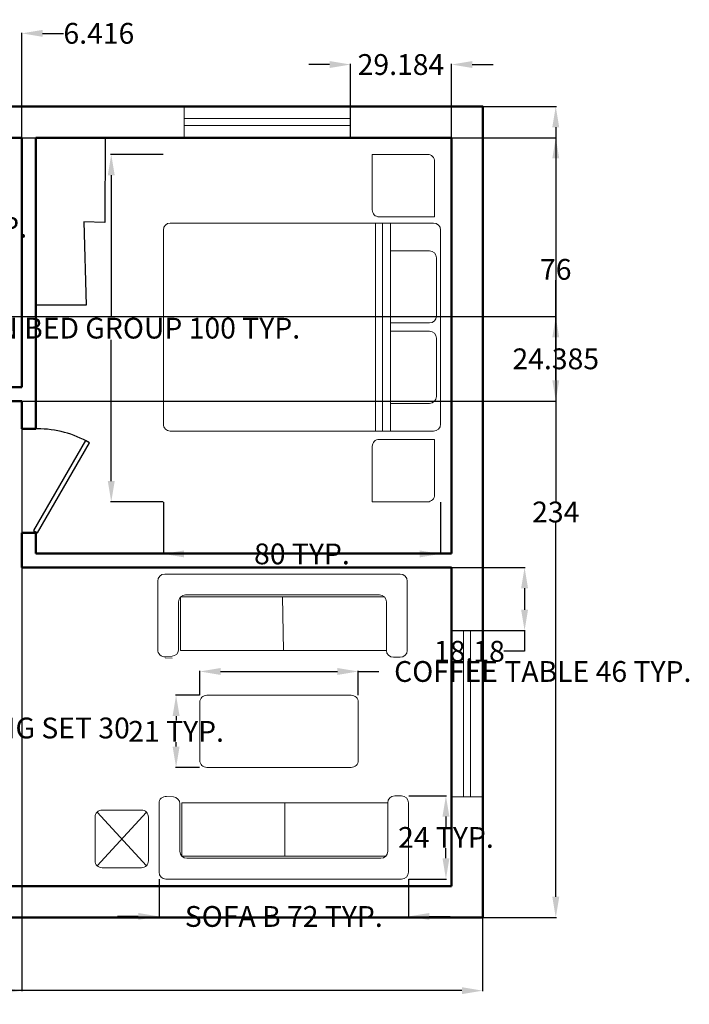
# Model space of a CAD drawing. Units: inches. Extents: x -22 to 471, y -231 to 53.
# Tile 3 of 3: x 277 to 471, y -231 to 53. Entities that reach past the tile are written whole.
import ezdxf

# ---------------------------------------------------------------- set-up
doc = ezdxf.new("R2010")
doc.units = ezdxf.units.IN
doc.header["$MEASUREMENT"] = 0
for name, color, linetype, lineweight in [('A-ANNO-DIMS', 2, 'Continuous', 18), ('A-DOOR', 3, 'Continuous', 25), ('A-FLOR-CASE', 32, 'Continuous', 25), ('A-FURN', 8, 'Continuous', 18), ('A-GLAZ', 4, 'Continuous', 18), ('A-WALL', 7, 'Continuous', 50)]:
    doc.layers.add(name, color=color, linetype=linetype, lineweight=lineweight)
doc.styles.get("Standard").update_dxf_attribs({"font": 'arial.ttf'})
doc.dimstyles.get("Standard").update_dxf_attribs({"dimtxt": 6, "dimasz": 6, "dimexe": 0.18, "dimexo": 0.0625, "dimgap": 0.09, "dimtad": 0, "dimtih": 1, "dimtoh": 1, "dimdec": 0, "dimzin": 0, "dimdsep": 46, "dimlunit": 4, "dimtxsty": 'Standard', "dimcen": 0.09, "dimadec": 0, "dimazin": 0, "dimtfac": 1, "dimtdec": 0, "dimtofl": 0, "dimtmove": 0, "dimatfit": 3, "dimfxl": 1, "dimtolj": 1, "dimtzin": 0, "dimarcsym": 0})

# ---------------------------------------------------------------- blocks, each defined once
blk = doc.blocks.new('Bed - Queen')
for p, q in [((2, 0), (58, 0)), ((0, -78), (0, -2)), ((10, -1.2), (26.8, -1.2)), ((33.2, -1.2), (50, -1.2)), ((60, -2), (60, -78)), ((8, -14.4), (8, -3.2)), ((28.8, -3.2), (28.8, -14.4)), ((31.2, -14.4), (31.2, -3.2)), ((52, -3.2), (52, -14.4)), ((0, -14.4), (60, -14.4)), ((60, -16.8), (0, -16.8)), ((60, -18.8), (0, -18.8)), ((58, -80), (2, -80))]:
    blk.add_line(p, q)
for points in [[(-17.8, -1.72), (-1.8, -1.72), (-1.8, -17.72, -0.414214), (-3.8, -19.72), (-19.8, -19.72), (-19.8, -3.72, -0.414214)], [(62.41, -1.72), (78.41, -1.72, -0.414214), (80.41, -3.72), (80.41, -19.72), (64.41, -19.72, -0.414214), (62.41, -17.72)]]:
    blk.add_lwpolyline(points, format="xyb", close=True)
for centre, start, end in [((2, -2), 90, 180), ((58, -2), 0, 90), ((10, -3.2), 90, 180), ((26.8, -3.2), 0, 90), ((33.2, -3.2), 90, 180), ((50, -3.2), 0, 90), ((2, -78), 180, 270), ((58, -78), 270, 0)]:
    blk.add_arc(centre, 2, start, end)
blk = doc.blocks.new('*U6')
for p, q in [((0, 0), (0, -6)), ((-40, 0), (-40, -6))]:
    blk.add_line(p, q)
blk.add_lwpolyline([(0, 0), (-34.64, 20), (-35.52, 18.48), (-0.88, -1.52)], close=True)
blk.add_arc((0, 0), 40, 150, 180)
blk = doc.blocks.new('WIN-48IN')
for p, q in [((0, 5.5), (48, 5.5)), ((0, 3.5), (48, 3.5))]:
    blk.add_line(p, q)
for points in [[(0, 0), (0, 9)], [(48, 9), (48, 0)]]:
    blk.add_lwpolyline(points)
blk = doc.blocks.new('SOFA-72IN-A')
for p, q in [((2, 24.28), (70, 24.28)), ((0, 2.42), (0, 22.28)), ((72, 22.28), (72, 2.28)), ((64, 18.28), (8, 18.28)), ((36.29, 2.28), (36, 17.7)), ((6, 16.28), (6, 2.56)), ((66, 2.28), (66, 16.28)), ((4.14, 0.57), (2.14, 0.43)), ((4.14, 0), (2.14, 0.14)), ((70, 0.28), (68, 0.28)), ((70, 0.28), (68, 0.28))]:
    blk.add_line(p, q)
blk.add_lwpolyline([(66, 16.28), (66, 2.28), (6.59, 2.28), (6.59, 17.7), (65.41, 17.7)])
for centre, start, end in [((2, 22.28), 90, 180), ((70, 22.28), 0, 90), ((8, 16.28), 90, 180), ((64, 16.28), 0, 90), ((2, 2.42), 180, 273.9184), ((4, 2.56), 273.9184, 0), ((68, 2.28), 180, 270), ((70, 2.28), 270, 0)]:
    blk.add_arc(centre, 2, start, end)
blk = doc.blocks.new('SOFA-72IN-B')
for p, q in [((2.14, 23.85), (4.14, 23.72)), ((68, 24), (70, 24)), ((0, 21.86), (0, 2)), ((6, 8), (6, 21.72)), ((36.29, 22), (36.29, 6.59)), ((66, 22), (66, 8)), ((72, 2), (72, 22)), ((64, 6), (8, 6)), ((2, 0), (70, 0))]:
    blk.add_line(p, q)
blk.add_lwpolyline([(66, 8), (66, 22), (6.59, 22), (6.59, 6.59), (65.41, 6.59)])
for centre, start, end in [((2, 21.86), 86.0816, 180), ((4, 21.72), 0, 86.0816), ((68, 22), 90, 180), ((70, 22), 0, 90), ((8, 8), 180, 270), ((64, 8), 270, 0), ((2, 2), 180, 270), ((70, 2), 270, 0)]:
    blk.add_arc(centre, 2, start, end)
blk = doc.blocks.new('TABLE-COFFEE')
blk.add_lwpolyline([(2, 20.83), (43.71, 20.83, -0.414214), (45.71, 18.83), (45.71, 2, -0.414214), (43.71, 0), (2, 0, -0.414214), (0, 2), (0, 18.83, -0.414214)], format="xyb", close=True)
blk = doc.blocks.new('TABLE-END')
for p, q in [((0.56, 0.61), (14.82, 16.04)), ((0.56, 16.04), (14.82, 0.61))]:
    blk.add_line(p, q)
blk.add_lwpolyline([(2, 16.65), (13.39, 16.65, -0.414214), (15.39, 14.65), (15.39, 2, -0.414214), (13.39, 0), (2, 0, -0.414214), (0, 2), (0, 14.65, -0.414214)], format="xyb", close=True)
blk = doc.blocks.new('BEDROOM-BUILTIN')
for p, q in [((0, 47.86), (0.1, 23.86)), ((0.1, 23.86), (6.1, 23.99)), ((6.1, 23.99), (5.51, 0)), ((5.51, 0), (20.03, 0))]:
    blk.add_line(p, q)
blk = doc.blocks.new('*D19')
at = {"layer": 'A-ANNO-DIMS', "color": 0, "lineweight": -2, "transparency": 16777216}
for p, q in [((318.71, 14.16), (303.56, 14.16)), ((303.74, 8.16), (303.74, -32.56)), ((303.74, -80.05), (303.74, -39.32)), ((318.71, -86.05), (303.56, -86.05))]:
    blk.add_line(p, q, dxfattribs=at)
at = {"layer": 'A-ANNO-DIMS', "color": 0, "transparency": 16777216}
for points in [[(302.74, 8.16), (304.74, 8.16), (303.74, 14.16)], [(302.74, -80.05), (304.74, -80.05), (303.74, -86.05)]]:
    blk.add_solid(points, dxfattribs=at)
at = {"layer": 'Defpoints', "color": 0, "transparency": 16777216}
for p in [(318.77, 14.16), (303.74, -86.05), (318.77, -86.05)]:
    blk.add_point(p, dxfattribs=at)
at = {"layer": 'A-ANNO-DIMS', "color": 0, "transparency": 16777216, "insert": (303.74, -35.94), "char_height": 6, "attachment_point": 5}
blk.add_mtext('\\A1;QUEEN BED GROUP 100 TYP.', dxfattribs=at)
blk = doc.blocks.new('*D20')
at = {"layer": 'A-ANNO-DIMS', "color": 0, "lineweight": -2, "transparency": 16777216}
for p, q in [((318.77, -86.11), (318.77, -101.26)), ((398.77, -86.11), (398.77, -101.26)), ((324.77, -101.08), (344.08, -101.08)), ((392.77, -101.08), (373.47, -101.08))]:
    blk.add_line(p, q, dxfattribs=at)
at = {"layer": 'A-ANNO-DIMS', "color": 0, "transparency": 16777216}
for points in [[(324.77, -100.08), (324.77, -102.08), (318.77, -101.08)], [(392.77, -100.08), (392.77, -102.08), (398.77, -101.08)]]:
    blk.add_solid(points, dxfattribs=at)
at = {"layer": 'Defpoints', "color": 0, "transparency": 16777216}
for p in [(318.77, -86.05), (398.77, -86.05), (398.77, -101.08)]:
    blk.add_point(p, dxfattribs=at)
at = {"layer": 'A-ANNO-DIMS', "color": 0, "transparency": 16777216, "insert": (358.77, -101.08), "char_height": 6, "attachment_point": 5}
blk.add_mtext('\\A1;80 TYP.', dxfattribs=at)
blk = doc.blocks.new('*D27')
at = {"layer": 'A-ANNO-DIMS', "color": 0, "lineweight": -2, "transparency": 16777216}
for p, q in [((216.44, -146.93), (216.44, -151.49)), ((246.08, -146.93), (246.08, -151.49)), ((222.44, -151.31), (240.08, -151.31)), ((246.08, -151.31), (252.08, -151.31))]:
    blk.add_line(p, q, dxfattribs=at)
at = {"layer": 'A-ANNO-DIMS', "color": 0, "transparency": 16777216}
for points in [[(222.44, -150.31), (222.44, -152.31), (216.44, -151.31)], [(240.08, -150.31), (240.08, -152.31), (246.08, -151.31)]]:
    blk.add_solid(points, dxfattribs=at)
at = {"layer": 'Defpoints', "color": 0, "transparency": 16777216}
for p in [(216.44, -146.86), (246.08, -146.86), (246.08, -151.31)]:
    blk.add_point(p, dxfattribs=at)
at = {"layer": 'A-ANNO-DIMS', "color": 0, "transparency": 16777216, "insert": (281.46, -151.31), "char_height": 6, "attachment_point": 5}
blk.add_mtext('\\A1;DINING SET 30', dxfattribs=at)
blk = doc.blocks.new('*D33')
at = {"layer": 'A-ANNO-DIMS', "color": 0, "lineweight": -2, "transparency": 16777216}
for p, q in [((317.53, -194.95), (317.53, -205.86)), ((389.53, -194.95), (389.53, -205.86)), ((311.53, -205.68), (305.53, -205.68)), ((395.53, -205.68), (401.53, -205.68))]:
    blk.add_line(p, q, dxfattribs=at)
at = {"layer": 'A-ANNO-DIMS', "color": 0, "transparency": 16777216}
for points in [[(311.53, -204.68), (311.53, -206.68), (317.53, -205.68)], [(395.53, -204.68), (395.53, -206.68), (389.53, -205.68)]]:
    blk.add_solid(points, dxfattribs=at)
at = {"layer": 'Defpoints', "color": 0, "transparency": 16777216}
for p in [(317.53, -194.88), (389.53, -194.88), (389.53, -205.68)]:
    blk.add_point(p, dxfattribs=at)
at = {"layer": 'A-ANNO-DIMS', "color": 0, "transparency": 16777216, "insert": (353.53, -205.68), "char_height": 6, "attachment_point": 5}
blk.add_mtext('\\A1;SOFA B 72 TYP.', dxfattribs=at)
blk = doc.blocks.new('*D34')
at = {"layer": 'A-ANNO-DIMS', "color": 0, "lineweight": -2, "transparency": 16777216}
for p, q in [((389.6, -170.88), (400.51, -170.88)), ((400.33, -176.88), (400.33, -179.78)), ((400.33, -188.88), (400.33, -185.99)), ((389.6, -194.88), (400.51, -194.88))]:
    blk.add_line(p, q, dxfattribs=at)
at = {"layer": 'A-ANNO-DIMS', "color": 0, "transparency": 16777216}
for points in [[(399.33, -176.88), (401.33, -176.88), (400.33, -170.88)], [(399.33, -188.88), (401.33, -188.88), (400.33, -194.88)]]:
    blk.add_solid(points, dxfattribs=at)
at = {"layer": 'Defpoints', "color": 0, "transparency": 16777216}
for p in [(389.53, -170.88), (400.33, -170.88), (389.53, -194.88)]:
    blk.add_point(p, dxfattribs=at)
at = {"layer": 'A-ANNO-DIMS', "color": 0, "transparency": 16777216, "insert": (400.33, -182.88), "char_height": 6, "attachment_point": 5}
blk.add_mtext('\\A1;24 TYP.', dxfattribs=at)
blk = doc.blocks.new('*D35')
at = {"layer": 'A-ANNO-DIMS', "color": 0, "lineweight": -2, "transparency": 16777216}
for p, q in [((329.31, -141.79), (329.31, -134.82)), ((335.31, -135), (369.01, -135)), ((375.01, -141.79), (375.01, -134.82)), ((375.01, -135), (381.01, -135))]:
    blk.add_line(p, q, dxfattribs=at)
at = {"layer": 'A-ANNO-DIMS', "color": 0, "transparency": 16777216}
for points in [[(335.31, -134), (335.31, -136), (329.31, -135)], [(369.01, -134), (369.01, -136), (375.01, -135)]]:
    blk.add_solid(points, dxfattribs=at)
at = {"layer": 'Defpoints', "color": 0, "transparency": 16777216}
for p in [(375.01, -135), (329.31, -141.86), (375.01, -141.86)]:
    blk.add_point(p, dxfattribs=at)
at = {"layer": 'A-ANNO-DIMS', "color": 0, "transparency": 16777216, "insert": (428.27, -135), "char_height": 6, "attachment_point": 5}
blk.add_mtext('\\A1;COFFEE TABLE 46 TYP.', dxfattribs=at)
blk = doc.blocks.new('*D36')
at = {"layer": 'A-ANNO-DIMS', "color": 0, "lineweight": -2, "transparency": 16777216}
for p, q in [((329.24, -141.86), (322.27, -141.86)), ((322.45, -147.86), (322.45, -149.17)), ((322.45, -156.68), (322.45, -155.37)), ((329.24, -162.68), (322.27, -162.68))]:
    blk.add_line(p, q, dxfattribs=at)
at = {"layer": 'A-ANNO-DIMS', "color": 0, "transparency": 16777216}
for points in [[(321.45, -147.86), (323.45, -147.86), (322.45, -141.86)], [(321.45, -156.68), (323.45, -156.68), (322.45, -162.68)]]:
    blk.add_solid(points, dxfattribs=at)
at = {"layer": 'Defpoints', "color": 0, "transparency": 16777216}
for p in [(322.45, -141.86), (329.31, -141.86), (329.31, -162.68)]:
    blk.add_point(p, dxfattribs=at)
at = {"layer": 'A-ANNO-DIMS', "color": 0, "transparency": 16777216, "insert": (322.45, -152.27), "char_height": 6, "attachment_point": 5}
blk.add_mtext('\\A1;21 TYP.', dxfattribs=at)
blk = doc.blocks.new('*D41')
at = {"layer": 'A-ANNO-DIMS', "color": 0, "lineweight": -2, "transparency": 16777216}
for p, q in [((238, 19.01), (245.86, 19.01)), ((245.68, 13.01), (245.68, -3.6)), ((245.68, -26.6), (245.68, -9.99)), ((238, -32.6), (245.86, -32.6))]:
    blk.add_line(p, q, dxfattribs=at)
at = {"layer": 'A-ANNO-DIMS', "color": 0, "transparency": 16777216}
for points in [[(244.68, 13.01), (246.68, 13.01), (245.68, 19.01)], [(244.68, -26.6), (246.68, -26.6), (245.68, -32.6)]]:
    blk.add_solid(points, dxfattribs=at)
at = {"layer": 'Defpoints', "color": 0, "transparency": 16777216}
for p in [(237.93, 19.01), (245.68, 19.01), (237.93, -32.6)]:
    blk.add_point(p, dxfattribs=at)
at = {"layer": 'A-ANNO-DIMS', "color": 0, "transparency": 16777216, "insert": (245.68, -6.8), "char_height": 6, "attachment_point": 5}
blk.add_mtext('\\A1;COUNTER 52 TYP.', dxfattribs=at)
blk = doc.blocks.new('*D43')
at = {"layer": 'A-ANNO-DIMS', "color": 0, "lineweight": -2, "transparency": 16777216}
for p, q in [((8.93, -206.05), (8.93, -227.27)), ((410.93, -206.05), (410.93, -227.27)), ((14.93, -227.09), (203.13, -227.09)), ((404.93, -227.09), (216.74, -227.09))]:
    blk.add_line(p, q, dxfattribs=at)
at = {"layer": 'A-ANNO-DIMS', "color": 0, "transparency": 16777216}
for points in [[(14.93, -226.09), (14.93, -228.09), (8.93, -227.09)], [(404.93, -226.09), (404.93, -228.09), (410.93, -227.09)]]:
    blk.add_solid(points, dxfattribs=at)
at = {"layer": 'Defpoints', "color": 0, "transparency": 16777216}
for p in [(8.93, -205.99), (410.93, -205.99), (410.93, -227.09)]:
    blk.add_point(p, dxfattribs=at)
at = {"layer": 'A-ANNO-DIMS', "color": 0, "transparency": 16777216, "insert": (209.93, -227.09), "char_height": 6, "attachment_point": 5}
blk.add_mtext('\\A1;402', dxfattribs=at)
blk = doc.blocks.new('*D44')
at = {"layer": 'A-ANNO-DIMS', "color": 0, "lineweight": -2, "transparency": 16777216}
for p, q in [((411, 28.01), (432.21, 28.01)), ((432.03, 22.01), (432.03, -85.83)), ((432.03, -199.99), (432.03, -92.14)), ((411, -205.99), (432.21, -205.99))]:
    blk.add_line(p, q, dxfattribs=at)
at = {"layer": 'A-ANNO-DIMS', "color": 0, "transparency": 16777216}
for points in [[(431.03, 22.01), (433.03, 22.01), (432.03, 28.01)], [(431.03, -199.99), (433.03, -199.99), (432.03, -205.99)]]:
    blk.add_solid(points, dxfattribs=at)
at = {"layer": 'Defpoints', "color": 0, "transparency": 16777216}
for p in [(410.93, 28.01), (410.93, -205.99), (432.03, -205.99)]:
    blk.add_point(p, dxfattribs=at)
at = {"layer": 'A-ANNO-DIMS', "color": 0, "transparency": 16777216, "insert": (432.03, -88.99), "char_height": 6, "attachment_point": 5}
blk.add_mtext('\\A1;234', dxfattribs=at)
blk = doc.blocks.new('*D47')
at = {"layer": 'A-ANNO-DIMS', "color": 0, "lineweight": -2, "transparency": 16777216}
for p, q in [((265.52, 49.11), (259.52, 49.11)), ((271.52, 28.07), (271.52, 49.29)), ((277.93, 19.07), (277.93, 49.29)), ((283.93, 49.11), (289.93, 49.11))]:
    blk.add_line(p, q, dxfattribs=at)
at = {"layer": 'A-ANNO-DIMS', "color": 0, "transparency": 16777216}
for points in [[(265.52, 50.11), (265.52, 48.11), (271.52, 49.11)], [(283.93, 50.11), (283.93, 48.11), (277.93, 49.11)]]:
    blk.add_solid(points, dxfattribs=at)
at = {"layer": 'Defpoints', "color": 0, "transparency": 16777216}
for p in [(277.93, 49.11), (271.52, 28.01), (277.93, 19.01)]:
    blk.add_point(p, dxfattribs=at)
at = {"layer": 'A-ANNO-DIMS', "color": 0, "transparency": 16777216, "insert": (300.16, 49.11), "char_height": 6, "attachment_point": 5}
blk.add_mtext('\\A1;6.416', dxfattribs=at)
blk = doc.blocks.new('*D48')
at = {"layer": 'A-ANNO-DIMS', "color": 0, "lineweight": -2, "transparency": 16777216}
for p, q in [((366.750151, 40.111163), (360.750151, 40.111163)), ((372.750151, 19.073663), (372.750151, 40.291163)), ((401.934447, 19.073663), (401.934447, 40.291163)), ((407.934447, 40.111163), (413.934447, 40.111163))]:
    blk.add_line(p, q, dxfattribs=at)
at = {"layer": 'A-ANNO-DIMS', "color": 0, "transparency": 16777216}
for points in [[(366.750151, 41.111163), (366.750151, 39.111163), (372.750151, 40.111163)], [(407.934447, 41.111163), (407.934447, 39.111163), (401.934447, 40.111163)]]:
    blk.add_solid(points, dxfattribs=at)
at = {"layer": 'Defpoints', "color": 0, "transparency": 16777216}
for p in [(401.934447, 40.111163), (372.750151, 19.011163), (401.934447, 19.011163)]:
    blk.add_point(p, dxfattribs=at)
at = {"layer": 'A-ANNO-DIMS', "color": 0, "transparency": 16777216, "insert": (387.342299, 40.111163), "char_height": 6, "attachment_point": 5}
blk.add_mtext('\\A1;29.184', dxfattribs=at)
blk = doc.blocks.new('*D55')
at = {"layer": 'A-ANNO-DIMS', "color": 0, "lineweight": -2, "transparency": 16777216}
for p, q in [((213.93, -32.67), (213.93, -227.27)), ((277.93, -57.05), (277.93, -227.27)), ((219.93, -227.09), (241.54, -227.09)), ((271.93, -227.09), (250.33, -227.09))]:
    blk.add_line(p, q, dxfattribs=at)
at = {"layer": 'A-ANNO-DIMS', "color": 0, "transparency": 16777216}
for points in [[(219.93, -226.09), (219.93, -228.09), (213.93, -227.09)], [(271.93, -226.09), (271.93, -228.09), (277.93, -227.09)]]:
    blk.add_solid(points, dxfattribs=at)
at = {"layer": 'Defpoints', "color": 0, "transparency": 16777216}
for p in [(213.93, -32.6), (277.93, -56.99), (277.93, -227.09)]:
    blk.add_point(p, dxfattribs=at)
at = {"layer": 'A-ANNO-DIMS', "color": 0, "transparency": 16777216, "insert": (245.93, -227.09), "char_height": 6, "attachment_point": 5}
blk.add_mtext('\\A1;64', dxfattribs=at)
blk = doc.blocks.new('*D58')
at = {"layer": 'A-ANNO-DIMS', "color": 0, "lineweight": -2, "transparency": 16777216}
for p, q in [((402, -104.99), (423.21, -104.99)), ((423.03, -110.99), (423.03, -117.17)), ((402, -123.17), (423.21, -123.17)), ((423.03, -123.17), (423.03, -129.17)), ((423.03, -129.17), (417.03, -129.17))]:
    blk.add_line(p, q, dxfattribs=at)
at = {"layer": 'A-ANNO-DIMS', "color": 0, "transparency": 16777216}
for points in [[(422.03, -110.99), (424.03, -110.99), (423.03, -104.99)], [(422.03, -117.17), (424.03, -117.17), (423.03, -123.17)]]:
    blk.add_solid(points, dxfattribs=at)
at = {"layer": 'Defpoints', "color": 0, "transparency": 16777216}
for p in [(401.93, -104.99), (401.93, -123.17), (423.03, -123.17)]:
    blk.add_point(p, dxfattribs=at)
at = {"layer": 'A-ANNO-DIMS', "color": 0, "transparency": 16777216, "insert": (407.1, -129.17), "char_height": 6, "attachment_point": 5}
blk.add_mtext('\\A1;18.18', dxfattribs=at)
blk = doc.blocks.new('*D63')
at = {"layer": 'A-ANNO-DIMS', "color": 0, "lineweight": -2, "transparency": 16777216}
for p, q in [((162.91, -32.6), (432.21, -32.6)), ((432.03, -38.6), (432.03, -41.64)), ((432.03, -50.99), (432.03, -47.95)), ((162.91, -56.99), (432.21, -56.99))]:
    blk.add_line(p, q, dxfattribs=at)
at = {"layer": 'A-ANNO-DIMS', "color": 0, "transparency": 16777216}
for points in [[(431.03, -38.6), (433.03, -38.6), (432.03, -32.6)], [(431.03, -50.99), (433.03, -50.99), (432.03, -56.99)]]:
    blk.add_solid(points, dxfattribs=at)
at = {"layer": 'Defpoints', "color": 0, "transparency": 16777216}
for p in [(162.85, -32.6), (432.03, -32.6), (162.85, -56.99)]:
    blk.add_point(p, dxfattribs=at)
at = {"layer": 'A-ANNO-DIMS', "color": 0, "transparency": 16777216, "insert": (432.03, -44.8), "char_height": 6, "attachment_point": 5}
blk.add_mtext('\\A1;24.385', dxfattribs=at)
blk = doc.blocks.new('*D64')
at = {"layer": 'A-ANNO-DIMS', "color": 0, "lineweight": -2, "transparency": 16777216}
for p, q in [((278, 19.01), (432.21, 19.01)), ((432.03, 13.01), (432.03, -15.84)), ((432.03, -50.99), (432.03, -22.14)), ((278, -56.99), (432.21, -56.99))]:
    blk.add_line(p, q, dxfattribs=at)
at = {"layer": 'A-ANNO-DIMS', "color": 0, "transparency": 16777216}
for points in [[(431.03, 13.01), (433.03, 13.01), (432.03, 19.01)], [(431.03, -50.99), (433.03, -50.99), (432.03, -56.99)]]:
    blk.add_solid(points, dxfattribs=at)
at = {"layer": 'Defpoints', "color": 0, "transparency": 16777216}
for p in [(277.93, 19.01), (432.03, 19.01), (277.93, -56.99)]:
    blk.add_point(p, dxfattribs=at)
at = {"layer": 'A-ANNO-DIMS', "color": 0, "transparency": 16777216, "insert": (432.03, -18.99), "char_height": 6, "attachment_point": 5}
blk.add_mtext('\\A1;76', dxfattribs=at)

msp = doc.modelspace()

# ---------------------------------------------------------------- linework, layer by layer
at = {"layer": 'A-WALL'}
for p, q in [((277.9344, 19.0112), (213.9344, 19.0112)), ((277.9344, -52.9888), (277.9344, 19.0112)), ((401.9344, 19.0112), (281.9344, 19.0112)), ((281.9344, -64.9888), (281.9344, 19.0112)), ((401.9344, -100.9888), (401.9344, 19.0112)), ((277.9344, -52.9888), (261.3964, -52.9888)), ((277.9344, -56.9888), (257.0189, -56.9888)), ((277.9344, -64.9888), (277.9344, -56.9888)), ((281.9344, -64.9888), (277.9344, -64.9888)), ((277.9344, -104.9888), (277.9344, -94.9888)), ((281.9344, -94.9888), (277.9344, -94.9888)), ((281.9344, -100.9888), (281.9344, -94.9888)), ((401.9344, -100.9888), (281.9344, -100.9888)), ((401.9344, -104.9888), (277.9344, -104.9888)), ((401.9344, -196.9888), (401.9344, -104.9888)), ((257.9344, -196.9888), (401.9344, -196.9888))]:
    msp.add_line(p, q, dxfattribs=at)
msp.add_lwpolyline([(257.9344, -205.9888), (410.9344, -205.9888), (410.9344, 28.0112), (200.9344, 28.0112)], dxfattribs=at)

# ---------------------------------------------------------------- block references
at = {"layer": 'A-DOOR', "xscale": 0.75, "yscale": 0.75, "zscale": 0.75, "rotation": 270}
msp.add_blockref('*U6', (282.4344, -94.9888), dxfattribs=at)
at = {"layer": 'A-FLOR-CASE', "extrusion": (0, 0, -1), "zscale": -1}
msp.add_blockref('BEDROOM-BUILTIN', (-301.9669, -29.2772), dxfattribs=at)
at = {"layer": 'A-FURN', "rotation": 270}
msp.add_blockref('Bed - Queen', (398.7741, -5.6372), dxfattribs=at)
at = {"layer": 'A-FURN'}
for name, p in [('SOFA-72IN-A', (317.1571, -131.187)), ('TABLE-COFFEE', (329.3051, -162.683)), ('SOFA-72IN-B', (317.5331, -194.884)), ('TABLE-END', (299.0811, -191.641))]:
    msp.add_blockref(name, p, dxfattribs=at)
at = {"layer": 'A-GLAZ'}
msp.add_blockref('WIN-48IN', (324.75, 19.011), dxfattribs=at)
at = {"layer": 'A-GLAZ', "rotation": 269.9999999999998}
msp.add_blockref('WIN-48IN', (401.9343, -123.1688), dxfattribs=at)

# ---------------------------------------------------------------- dimensions: what is measured, and where the dimension line sits
at = {"layer": 'A-ANNO-DIMS'}
for base, p1, p2, override, picture, middle in [((277.9344, 49.1112), (271.5183, 28.0112), (277.9344, 19.0112), {"dimdec": 3, "dimlfac": 1, "dimrnd": 0, "dimzin": 0, "dimdsep": 46, "dimlunit": 2}, '*D47', (300.1622, 49.1112)), ((401.9344, 40.1112), (372.7502, 19.0112), (401.9344, 19.0112), {"dimdec": 3, "dimlfac": 1, "dimrnd": 0, "dimzin": 0, "dimdsep": 46, "dimlunit": 2}, '*D48', (387.3423, 40.1112)), ((277.9344, -227.0888), (213.9344, -32.6035), (277.9344, -56.9888), {"dimdec": 0, "dimlfac": 1, "dimrnd": 0, "dimzin": 0, "dimdsep": 46, "dimlunit": 2}, '*D55', (245.9344, -227.0888)), ((410.9344, -227.0888), (8.9344, -205.9888), (410.9344, -205.9888), {"dimdec": 0, "dimlfac": 1, "dimrnd": 0, "dimzin": 0, "dimdsep": 46, "dimlunit": 2}, '*D43', (209.9344, -227.0888))]:
    dim = msp.add_linear_dim(base=base, p1=p1, p2=p2, dimstyle='Standard', override=override, dxfattribs=at)
    dim.commit()
    dim.dimension.update_dxf_attribs({"geometry": picture, "text_midpoint": middle})
for base, p1, p2, angle, override, picture, middle in [((432.0344, -205.9888), (410.9344, 28.0112), (410.9344, -205.9888), 90, {"dimdec": 0, "dimlfac": 1, "dimrnd": 0, "dimzin": 0, "dimdsep": 46, "dimlunit": 2}, '*D44', (432.0344, -88.9888)), ((432.0344, 19.0112), (277.9344, -56.9888), (277.9344, 19.0112), 90, {"dimdec": 0, "dimlfac": 1, "dimrnd": 0, "dimzin": 0, "dimdsep": 46, "dimlunit": 2}, '*D64', (432.0344, -18.9888)), ((432.0344, -32.6035), (162.85, -56.9888), (162.85, -32.6035), 90, {"dimdec": 3, "dimlfac": 1, "dimrnd": 0, "dimzin": 0, "dimdsep": 46, "dimlunit": 2}, '*D63', (432.0344, -44.7962)), ((423.0344, -123.1689), (401.9344, -104.9888), (401.9344, -123.1689), 270, {"dimdec": 2, "dimlfac": 1, "dimrnd": 0, "dimzin": 0, "dimdsep": 46, "dimlunit": 2}, '*D58', (407.0972, -129.1689))]:
    dim = msp.add_linear_dim(base=base, p1=p1, p2=p2, angle=angle, dimstyle='Standard', override=override, dxfattribs=at)
    dim.commit()
    dim.dimension.update_dxf_attribs({"geometry": picture, "text_midpoint": middle})
for base, p1, p2, angle, text, picture, middle in [((245.6766, 19.0112), (237.9344, -32.6035), (237.9344, 19.0112), 90, 'COUNTER <> TYP.', '*D41', (245.6766, -6.7962)), ((303.7424, -86.0462), (318.774, 14.1648), (318.774, -86.0462), 270, 'QUEEN BED GROUP <> TYP.', '*D19', (303.7424, -35.9407)), ((322.4491, -141.8568), (329.3051, -162.6829), (329.3051, -141.8568), 90, '<> TYP.', '*D36', (322.4491, -152.2699)), ((400.3328, -170.8839), (389.5328, -194.8839), (389.5328, -170.8839), 90, '<> TYP.', '*D34', (400.3328, -182.8839))]:
    dim = msp.add_linear_dim(base=base, p1=p1, p2=p2, angle=angle, text=text, dimstyle='Standard', override={"dimdec": 0, "dimlfac": 1, "dimrnd": 0, "dimzin": 0, "dimdsep": 46, "dimlunit": 2}, dxfattribs=at)
    dim.commit()
    dim.dimension.update_dxf_attribs({"geometry": picture, "text_midpoint": middle})
for base, p1, p2, text, picture, middle in [((398.7741, -101.0779), (318.774, -86.0462), (398.7741, -86.0462), '<> TYP.', '*D20', (358.7741, -101.0779)), ((375.0114, -135.0009), (329.3051, -141.8568), (375.0114, -141.8568), 'COFFEE TABLE <> TYP.', '*D35', (428.2726, -135.0009)), ((246.08, -151.3091), (216.4404, -146.8631), (246.08, -146.8631), 'DINING SET <>', '*D27', (281.4558, -151.3091)), ((389.5328, -205.6839), (317.5328, -194.8839), (389.5328, -194.8839), 'SOFA B <> TYP.', '*D33', (353.5328, -205.6839))]:
    dim = msp.add_linear_dim(base=base, p1=p1, p2=p2, text=text, dimstyle='Standard', override={"dimdec": 0, "dimlfac": 1, "dimrnd": 0, "dimzin": 0, "dimdsep": 46, "dimlunit": 2}, dxfattribs=at)
    dim.commit()
    dim.dimension.update_dxf_attribs({"geometry": picture, "text_midpoint": middle})

doc.saveas('drawing.dxf')
